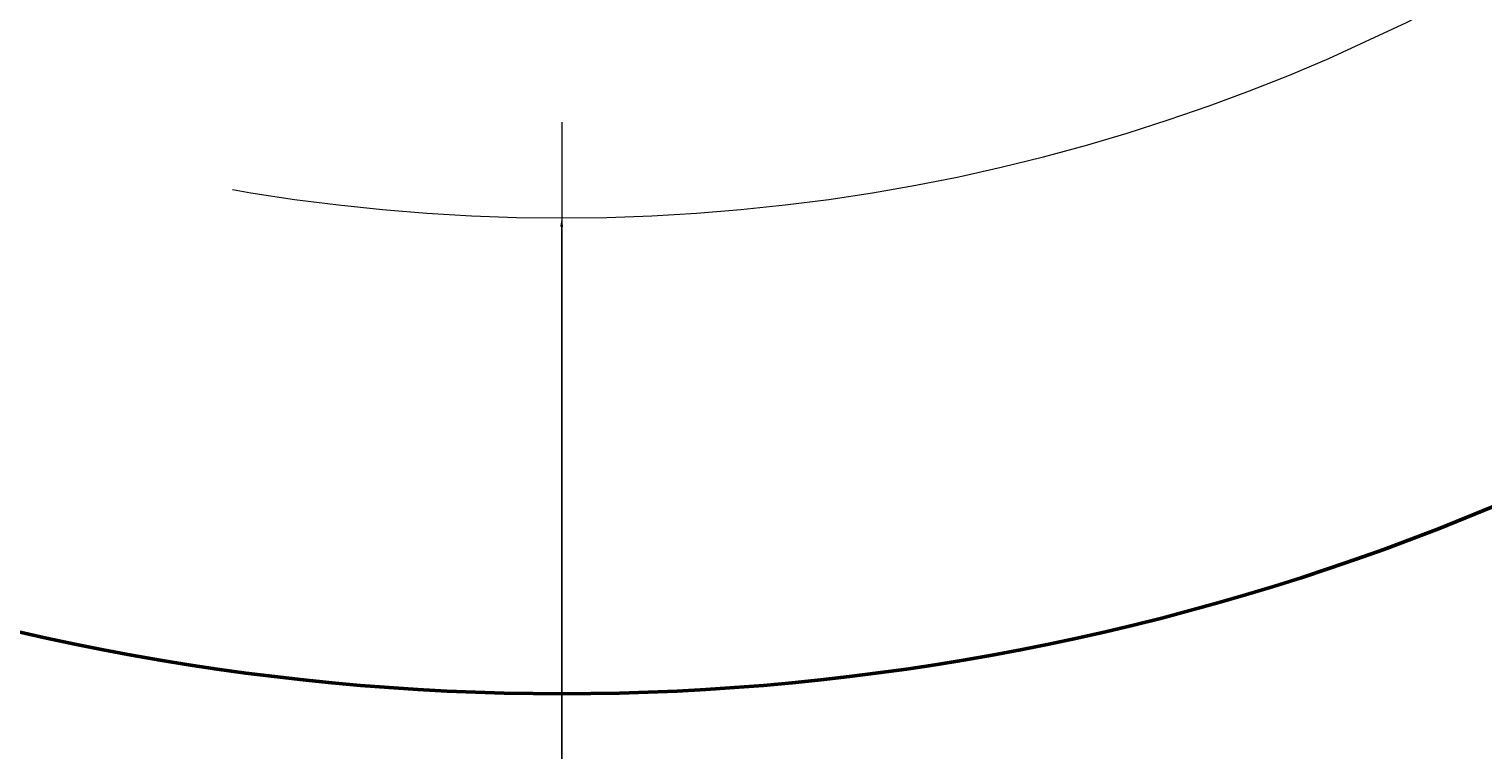
# Model space of a CAD drawing. Units: millimetres. Extents: x -53 to 92, y -147 to 37.
# Tile 4 of 16: x 8 to 38, y -105 to -90. Entities that reach past the tile are written whole.
import ezdxf

# ---------------------------------------------------------------- set-up
doc = ezdxf.new("R2010")
doc.units = ezdxf.units.MM
doc.header["$MEASUREMENT"] = 0
doc.linetypes.add('CENTER', pattern=[50.8, 31.75, -6.35, 6.35, -6.35])
for name, color, linetype, lineweight in [('M-CNTR', 4, 'CENTER', 18), ('M-DIMS', 2, 'Continuous', 25), ('M-OUTL', 7, 'Continuous', 50)]:
    doc.layers.add(name, color=color, linetype=linetype, lineweight=lineweight)
doc.styles.get("Standard").update_dxf_attribs({"font": 'arial.ttf'})
doc.dimstyles.get("Standard").update_dxf_attribs({"dimtxt": 0.18, "dimasz": 0.18, "dimexe": 0.18, "dimexo": 0.0625, "dimgap": 0.09, "dimtad": 0, "dimtih": 1, "dimtoh": 1, "dimdec": 4, "dimzin": 0, "dimdsep": 46, "dimtxsty": 'Standard', "dimcen": 0.09, "dimadec": 0, "dimazin": 0, "dimtfac": 1, "dimtdec": 4, "dimtofl": 0, "dimtmove": 0, "dimatfit": 3, "dimfxl": 1, "dimtolj": 1, "dimtzin": 0, "dimarcsym": 0})

# ---------------------------------------------------------------- blocks, each defined once
blk = doc.blocks.new('*D16')
at = {"layer": 'Defpoints', "color": 0, "transparency": 16777216}
for p in [(-22.056, -94.992), (59.969, -94.992), (59.969, -138.812)]:
    blk.add_point(p, dxfattribs=at)
at = {"layer": 'M-DIMS', "color": 0, "lineweight": -2, "transparency": 16777216}
for p, q in [((-22.056, -95.055), (-22.056, -138.992)), ((59.969, -95.055), (59.969, -138.992)), ((-21.876, -138.812), (18.563, -138.812)), ((59.789, -138.812), (19.349, -138.812))]:
    blk.add_line(p, q, dxfattribs=at)
at = {"layer": 'M-DIMS', "color": 0, "transparency": 16777216}
for points in [[(-21.876, -138.782), (-21.876, -138.842), (-22.056, -138.812)], [(59.789, -138.782), (59.789, -138.842), (59.969, -138.812)]]:
    blk.add_solid(points, dxfattribs=at)
at = {"layer": 'M-DIMS', "color": 0, "transparency": 16777216, "insert": (18.956, -138.812), "char_height": 0.18, "attachment_point": 5}
blk.add_mtext('\\A1;82.02', dxfattribs=at)
blk = doc.blocks.new('*D17')
at = {"layer": 'Defpoints', "color": 0, "transparency": 16777216}
for p in [(-46.81, 25.909), (28.564, 25.909), (18.165, -111.975)]:
    blk.add_point(p, dxfattribs=at)
at = {"layer": 'M-DIMS', "color": 0, "lineweight": -2, "transparency": 16777216}
for p, q in [((28.502, 25.909), (-46.99, 25.909)), ((-46.81, 25.729), (-46.81, -42.851)), ((-46.81, -111.795), (-46.81, -43.215)), ((18.102, -111.975), (-46.99, -111.975))]:
    blk.add_line(p, q, dxfattribs=at)
at = {"layer": 'M-DIMS', "color": 0, "transparency": 16777216}
for points in [[(-46.84, 25.729), (-46.78, 25.729), (-46.81, 25.909)], [(-46.84, -111.795), (-46.78, -111.795), (-46.81, -111.975)]]:
    blk.add_solid(points, dxfattribs=at)
at = {"layer": 'M-DIMS', "color": 0, "transparency": 16777216, "insert": (-46.81, -43.033), "char_height": 0.18, "attachment_point": 5}
blk.add_mtext('\\A1;137.88', dxfattribs=at)
blk = doc.blocks.new('*D18')
at = {"layer": 'Defpoints', "color": 0, "transparency": 16777216}
for p in [(19.753, 4.014), (18.16, -111.975)]:
    blk.add_point(p, dxfattribs=at)
at = {"layer": 'M-DIMS', "color": 0, "lineweight": -2, "transparency": 16777216}
for p, q in [((18.866, -53.98), (19.046, -53.98)), ((18.956, -54.07), (18.956, -53.89)), ((17.682, -146.771), (18.158, -112.155)), ((17.502, -146.771), (17.682, -146.771))]:
    blk.add_line(p, q, dxfattribs=at)
at = {"layer": 'M-DIMS', "color": 0, "transparency": 16777216}
blk.add_solid([(18.128, -112.154), (18.188, -112.155), (18.16, -111.975)], dxfattribs=at)
at = {"layer": 'M-DIMS', "color": 0, "transparency": 16777216, "insert": (17.115, -146.771), "char_height": 0.18, "attachment_point": 5}
blk.add_mtext('\\A1;∅116', dxfattribs=at)
blk = doc.blocks.new('*D23')
at = {"layer": 'Defpoints', "color": 0, "transparency": 16777216}
for p in [(18.956, -54.07), (18.954, -94.07)]:
    blk.add_point(p, dxfattribs=at)
at = {"layer": 'M-DIMS', "color": 0, "lineweight": -2, "transparency": 16777216}
for p, q in [((18.866, -54.07), (19.046, -54.07)), ((18.956, -54.16), (18.956, -53.98)), ((18.953, -118.07), (18.954, -94.25)), ((18.773, -118.07), (18.953, -118.07))]:
    blk.add_line(p, q, dxfattribs=at)
at = {"layer": 'M-DIMS', "color": 0, "transparency": 16777216}
blk.add_solid([(18.924, -94.25), (18.984, -94.25), (18.954, -94.07)], dxfattribs=at)
at = {"layer": 'M-DIMS', "color": 0, "transparency": 16777216, "insert": (18.468, -118.07), "char_height": 0.18, "attachment_point": 5}
blk.add_mtext('\\A1;R40', dxfattribs=at)
blk = doc.blocks.new('*D24')
at = {"layer": 'Defpoints', "color": 0, "transparency": 16777216}
for p in [(18.956, -53.969), (2.002, -101.015)]:
    blk.add_point(p, dxfattribs=at)
at = {"layer": 'M-DIMS', "color": 0, "lineweight": -2, "transparency": 16777216}
for p, q in [((18.956, -54.059), (18.956, -53.879)), ((18.866, -53.969), (19.046, -53.969)), ((-8.171, -129.243), (1.941, -101.184)), ((-8.351, -129.243), (-8.171, -129.243))]:
    blk.add_line(p, q, dxfattribs=at)
at = {"layer": 'M-DIMS', "color": 0, "transparency": 16777216}
blk.add_solid([(1.912, -101.174), (1.969, -101.195), (2.002, -101.015)], dxfattribs=at)
at = {"layer": 'M-DIMS', "color": 0, "transparency": 16777216, "insert": (-8.813, -129.243), "char_height": 0.18, "attachment_point": 5}
blk.add_mtext('\\A1;R50.01', dxfattribs=at)

msp = doc.modelspace()

# ---------------------------------------------------------------- linework, layer by layer
at = {"layer": 'M-CNTR'}
msp.add_line((18.95638, -53.98007), (18.95638, -130.36235), dxfattribs=at)
msp.add_arc((18.95638, -54.07007), 40, 187.365915, 352.627832, dxfattribs=at)
at = {"layer": 'M-OUTL'}
for centre, radius, start, end in [((18.95638, -53.98007), 58, 108.3895553, 70.0459142), ((18.95621, -53.96903), 50.00792, 225.009078, 314.99431)]:
    msp.add_arc(centre, radius, start, end, dxfattribs=at)

# ---------------------------------------------------------------- dimensions: what is measured, and where the dimension line sits
at = {"layer": 'M-DIMS'}
dim = msp.add_linear_dim(base=(-46.8103, 25.90924), p1=(18.16452, -111.97467), p2=(28.56407, 25.90924), angle=90, dimstyle='Standard', override={"dimdec": 2, "dimlfac": 1, "dimrnd": 0, "dimzin": 0, "dimdsep": 46, "dimlunit": 2}, dxfattribs=at)
dim.commit()
dim.dimension.update_dxf_attribs({"geometry": '*D17', "text_midpoint": (-46.8103, -43.03271)})
dim = msp.add_diameter_dim_2p(p1=(19.75275, 4.01446), p2=(18.16001, -111.9746), dimstyle='Standard', override={"dimdec": 0, "dimlfac": 1, "dimrnd": 0, "dimzin": 0, "dimdsep": 46, "dimlunit": 2}, dxfattribs=at)
dim.commit()
dim.dimension.update_dxf_attribs({"geometry": '*D18', "text_midpoint": (17.11548, -146.77132), "dimtype": 163})
for center, mpoint, override, picture, middle in [((18.95621, -53.96903), (2.00175, -101.01516), {"dimdec": 2, "dimlfac": 1, "dimrnd": 0, "dimzin": 0, "dimdsep": 46, "dimlunit": 2}, '*D24', (-8.8134, -129.24283)), ((18.95638, -54.07007), (18.954, -94.07007), {"dimdec": 0, "dimlfac": 1, "dimrnd": 0, "dimzin": 0, "dimdsep": 46, "dimlunit": 2}, '*D23', (18.46782, -118.07007))]:
    dim = msp.add_radius_dim(center=center, mpoint=mpoint, dimstyle='Standard', override=override, dxfattribs=at)
    dim.commit()
    dim.dimension.update_dxf_attribs({"geometry": picture, "text_midpoint": middle, "dimtype": 164})
dim = msp.add_linear_dim(base=(59.96857, -138.81235), p1=(-22.0558, -94.99225), p2=(59.96857, -94.99226), dimstyle='Standard', override={"dimdec": 2, "dimlfac": 1, "dimrnd": 0, "dimzin": 0, "dimdsep": 46, "dimlunit": 2}, dxfattribs=at)
dim.commit()
dim.dimension.update_dxf_attribs({"geometry": '*D16', "text_midpoint": (18.95639, -138.81235)})

doc.saveas('drawing.dxf')
